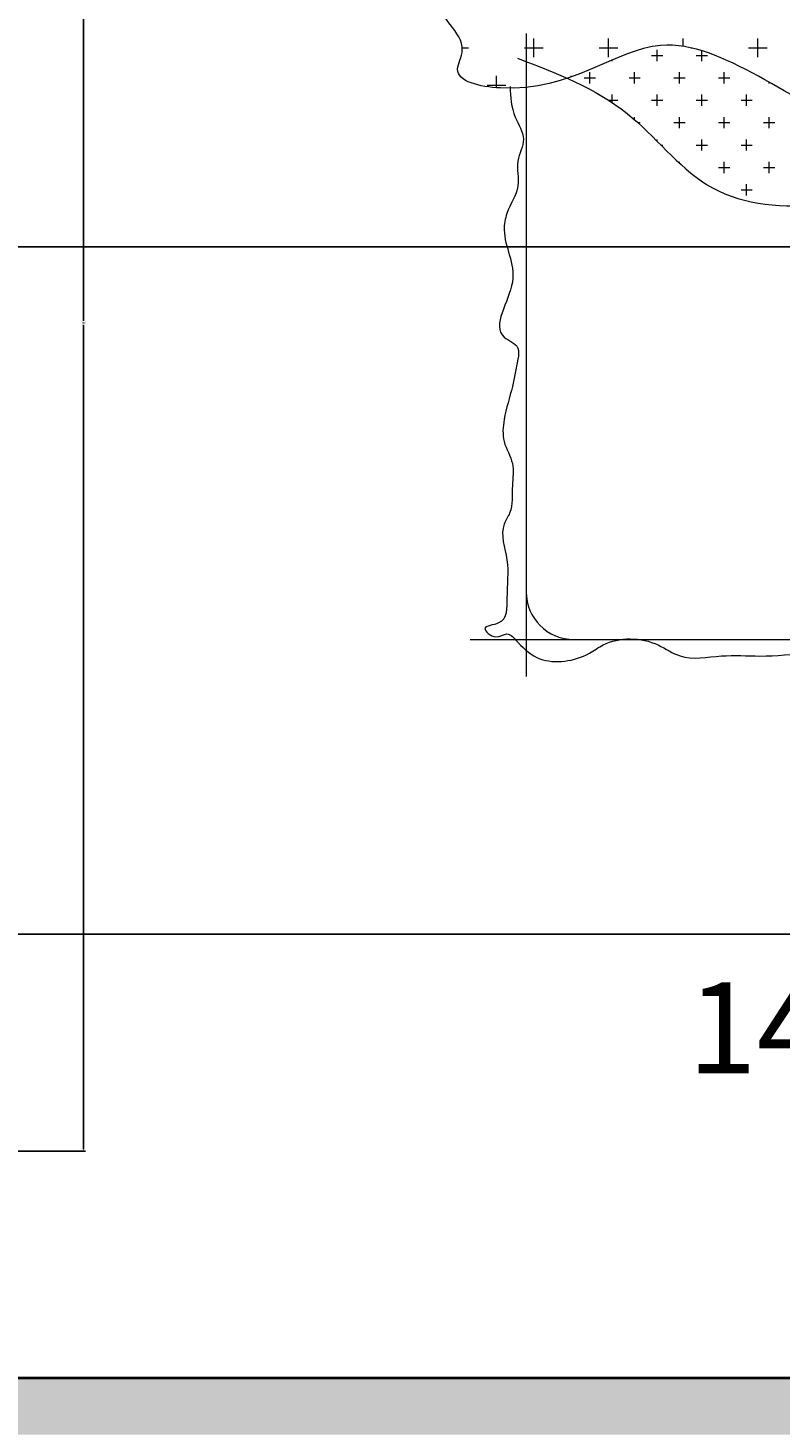
# Model space of a CAD drawing. Units: inches. Extents: x 2330 to 3943, y 1763 to 3461.
# Tile 31 of 40: x 3281 to 3347, y 2975 to 3098. Entities that reach past the tile are written whole.
import ezdxf

# ---------------------------------------------------------------- set-up
doc = ezdxf.new("R2010")
doc.units = ezdxf.units.IN
for name, color, linetype, lineweight in [('A-ANNO-DIMS', 2, 'Continuous', 18), ('A-AREA-IDEN', 7, 'Continuous', 18), ('A-FURN', 8, 'Continuous', 13), ('A-WALL', 7, 'Continuous', 40), ('A-WALL-PATT', 252, 'Continuous', 13)]:
    doc.layers.add(name, color=color, linetype=linetype, lineweight=lineweight)
doc.styles.get("Standard").update_dxf_attribs({"font": 'arial.ttf'})
doc.dimstyles.get("Standard").update_dxf_attribs({"dimtxt": 0.18, "dimasz": 0.18, "dimexe": 0.18, "dimexo": 0.0625, "dimgap": 0.09, "dimtad": 0, "dimtih": 1, "dimtoh": 1, "dimdec": 4, "dimzin": 0, "dimdsep": 46, "dimtxsty": 'Standard', "dimcen": 0.09, "dimadec": 0, "dimazin": 0, "dimtfac": 1, "dimtdec": 4, "dimtofl": 0, "dimtmove": 0, "dimatfit": 3, "dimfxl": 1, "dimtolj": 1, "dimtzin": 0, "dimarcsym": 0})

# ---------------------------------------------------------------- blocks, each defined once
blk = doc.blocks.new('A$C200C7901')
for p, q in [((0.5, 1.3845), (0.5, 0.3086)), ((0.3931, 1.3602), (0.4035, 1.3602)), ((0.3931, 1.3602), (0.4035, 1.3602)), ((0.4972, 1.3602), (0.5285, 1.3602)), ((0.4972, 1.3602), (0.5285, 1.3602)), ((0.4504, 1.2936), (0.4504, 1.3133)), ((0.4504, 1.2936), (0.4504, 1.3133)), ((0.4347, 1.2977), (0.466, 1.2977)), ((0.4347, 1.2977), (0.466, 1.2977)), ((0.4061, 0.3703), (2.0386, 0.3703))]:
    blk.add_line(p, q)
at = {"linetype": 'ByBlock'}
for p, q in [((0.5129, 1.3445), (0.5129, 1.3758)), ((0.5129, 1.3445), (0.5129, 1.3758)), ((0.6222, 1.3602), (0.6535, 1.3602)), ((0.6222, 1.3602), (0.6535, 1.3602)), ((0.6379, 1.3445), (0.6379, 1.3758)), ((0.6379, 1.3445), (0.6379, 1.3758)), ((0.7629, 1.3627), (0.7629, 1.3758)), ((0.7629, 1.3627), (0.7629, 1.3758)), ((0.7762, 1.3602), (0.7785, 1.3602)), ((0.7762, 1.3602), (0.7785, 1.3602)), ((0.8722, 1.3602), (0.9035, 1.3602)), ((0.8722, 1.3602), (0.9035, 1.3602)), ((0.8879, 1.3445), (0.8879, 1.3758)), ((0.8879, 1.3445), (0.8879, 1.3758)), ((0.6441, 1.3383), (0.6441, 1.3399)), ((0.6441, 1.3383), (0.6441, 1.3399)), ((0.7097, 1.3477), (0.7285, 1.3477)), ((0.7097, 1.3477), (0.7285, 1.3477)), ((0.7191, 1.3383), (0.7191, 1.357)), ((0.7191, 1.3383), (0.7191, 1.357)), ((0.7847, 1.3477), (0.8035, 1.3477)), ((0.7847, 1.3477), (0.8035, 1.3477)), ((0.7941, 1.3383), (0.7941, 1.3554)), ((0.7941, 1.3383), (0.7941, 1.3554)), ((0.5754, 1.3115), (0.5754, 1.3133)), ((0.5754, 1.3115), (0.5754, 1.3133)), ((0.6066, 1.3008), (0.6066, 1.3195)), ((0.6066, 1.3008), (0.6066, 1.3195)), ((0.6816, 1.3008), (0.6816, 1.3195)), ((0.6816, 1.3008), (0.6816, 1.3195)), ((0.7566, 1.3008), (0.7566, 1.3195)), ((0.7566, 1.3008), (0.7566, 1.3195)), ((0.8316, 1.3008), (0.8316, 1.3195)), ((0.8316, 1.3008), (0.8316, 1.3195)), ((0.5972, 1.3102), (0.616, 1.3102)), ((0.5972, 1.3102), (0.616, 1.3102)), ((0.6722, 1.3102), (0.691, 1.3102)), ((0.6722, 1.3102), (0.691, 1.3102)), ((0.7472, 1.3102), (0.766, 1.3102)), ((0.7472, 1.3102), (0.766, 1.3102)), ((0.8222, 1.3102), (0.841, 1.3102)), ((0.8222, 1.3102), (0.841, 1.3102)), ((0.9066, 1.3008), (0.9066, 1.3028)), ((0.9066, 1.3008), (0.9066, 1.3028)), ((0.6379, 1.2727), (0.6535, 1.2727)), ((0.6379, 1.2727), (0.6535, 1.2727)), ((0.6441, 1.2686), (0.6441, 1.282)), ((0.6441, 1.2686), (0.6441, 1.282)), ((0.7097, 1.2727), (0.7285, 1.2727)), ((0.7097, 1.2727), (0.7285, 1.2727)), ((0.7191, 1.2633), (0.7191, 1.282)), ((0.7191, 1.2633), (0.7191, 1.282)), ((0.7847, 1.2727), (0.8035, 1.2727)), ((0.7847, 1.2727), (0.8035, 1.2727)), ((0.7941, 1.2633), (0.7941, 1.282)), ((0.7941, 1.2633), (0.7941, 1.282)), ((0.8597, 1.2727), (0.8785, 1.2727)), ((0.8597, 1.2727), (0.8785, 1.2727)), ((0.8691, 1.2633), (0.8691, 1.282)), ((0.8691, 1.2633), (0.8691, 1.282)), ((0.6816, 1.2398), (0.6816, 1.2445)), ((0.6816, 1.2398), (0.6816, 1.2445)), ((0.7566, 1.2258), (0.7566, 1.2445)), ((0.7566, 1.2258), (0.7566, 1.2445)), ((0.8316, 1.2258), (0.8316, 1.2445)), ((0.8316, 1.2258), (0.8316, 1.2445)), ((0.9066, 1.2258), (0.9066, 1.2445)), ((0.9066, 1.2258), (0.9066, 1.2445)), ((0.6868, 1.2352), (0.691, 1.2352)), ((0.6868, 1.2352), (0.691, 1.2352)), ((0.7472, 1.2352), (0.766, 1.2352)), ((0.7472, 1.2352), (0.766, 1.2352)), ((0.8222, 1.2352), (0.841, 1.2352)), ((0.8222, 1.2352), (0.841, 1.2352)), ((0.8972, 1.2352), (0.916, 1.2352)), ((0.8972, 1.2352), (0.916, 1.2352)), ((0.7191, 1.2041), (0.7191, 1.207)), ((0.7191, 1.2041), (0.7191, 1.207)), ((0.7255, 1.1977), (0.7285, 1.1977)), ((0.7255, 1.1977), (0.7285, 1.1977)), ((0.7847, 1.1977), (0.8035, 1.1977)), ((0.7847, 1.1977), (0.8035, 1.1977)), ((0.7941, 1.1883), (0.7941, 1.207)), ((0.7941, 1.1883), (0.7941, 1.207)), ((0.8597, 1.1977), (0.8785, 1.1977)), ((0.8597, 1.1977), (0.8785, 1.1977)), ((0.8691, 1.1883), (0.8691, 1.207)), ((0.8691, 1.1883), (0.8691, 1.207)), ((0.7566, 1.1674), (0.7566, 1.1695)), ((0.7566, 1.1674), (0.7566, 1.1695)), ((0.7646, 1.1602), (0.766, 1.1602)), ((0.7646, 1.1602), (0.766, 1.1602)), ((0.8222, 1.1602), (0.841, 1.1602)), ((0.8222, 1.1602), (0.841, 1.1602)), ((0.8316, 1.1508), (0.8316, 1.1695)), ((0.8316, 1.1508), (0.8316, 1.1695)), ((0.8972, 1.1602), (0.916, 1.1602)), ((0.8972, 1.1602), (0.916, 1.1602)), ((0.9066, 1.1508), (0.9066, 1.1695)), ((0.9066, 1.1508), (0.9066, 1.1695)), ((0.8691, 1.1133), (0.8691, 1.132)), ((0.8691, 1.1133), (0.8691, 1.132)), ((0.8597, 1.1227), (0.8785, 1.1227)), ((0.8597, 1.1227), (0.8785, 1.1227))]:
    blk.add_line(p, q, dxfattribs=at)
blk.add_arc((0.58, 0.4503), 0.08, 180, 270)
for points, knots in [([(0.4485, 1.7835), (0.4321, 1.7496), (0.4062, 1.6964), (0.49, 1.6713), (0.4719, 1.5969), (0.4123, 1.592), (0.4233, 1.5337), (0.4954, 1.5086), (0.4012, 1.4738), (0.3253, 1.4306), (0.4113, 1.3764), (0.3688, 1.3065), (0.5579, 1.2663), (0.741, 1.4533), (1.1127, 1.1109), (1.4811, 1.2478), (1.7885, 1.3492), (2.0357, 1.1637), (2.0748, 1.2974), (2.0876, 1.349), (2.0192, 1.3805), (2.0564, 1.4298), (2.0588, 1.4846), (1.9759, 1.5349), (2.1004, 1.5845), (2.0397, 1.6519), (1.971, 1.7053), (2.1104, 1.8981), (1.5946, 1.7967), (1.2448, 1.7472), (0.8129, 1.7935), (0.4953, 1.8548), (0.4582, 1.7983), (0.4485, 1.7835)], [0, 0, 0, 0, 88.420092, 139.08588, 204.302936, 239.695496, 287.801042, 327.365471, 412.960499, 463.626286, 552.059846, 584.668336, 662.614915, 940.993281, 1309.926334, 1844.022653, 1996.276242, 2316.43048, 2341.441004, 2404.707416, 2449.463774, 2514.680778, 2538.40571, 2613.031547, 2697.13096, 2760.903931, 2822.692699, 2945.47, 3215.060018, 3725.584917, 4361.974444, 4504.671998, 4555.32777, 4555.32777, 4555.32777, 4555.32777]), ([(0.4856, 1.3429), (0.5504, 1.3182), (0.6715, 1.2721), (0.8374, 1.0498), (1.1164, 1.1183), (1.3878, 1.1816), (1.5888, 1.1102), (1.8403, 1.1127), (1.9415, 1.2178), (2.0032, 1.2819)], [0, 0, 0, 0, 205.411753, 383.654933, 772.067458, 921.644661, 1226.793228, 1388.983508, 1642.292305, 1642.292305, 1642.292305, 1642.292305])]:
    blk.add_open_spline(points, degree=3, knots=knots)
blk.add_open_spline([(0.473, 1.2954), (0.4739, 1.2781), (0.4755, 1.2477), (0.5032, 1.2084), (0.4801, 1.1701), (0.4928, 1.1255), (0.4674, 1.0912), (0.4579, 1.0351), (0.501, 0.9724), (0.4311, 0.8832), (0.4902, 0.8637), (0.4843, 0.8288), (0.4774, 0.7906), (0.4625, 0.7457), (0.459, 0.6999), (0.4816, 0.6664), (0.4748, 0.625), (0.4791, 0.5889), (0.4533, 0.5528), (0.4738, 0.5004), (0.4658, 0.4502), (0.4696, 0.3946), (0.4189, 0.3935), (0.4493, 0.3684), (0.4694, 0.3857), (0.4922, 0.3576), (0.5297, 0.3262), (0.5917, 0.3353), (0.6454, 0.3754), (0.7083, 0.3741), (0.7643, 0.3328), (0.826, 0.346), (0.925, 0.3388), (1.0353, 0.3593), (1.1561, 0.3744), (1.2477, 0.3154), (1.3302, 0.3474), (1.4086, 0.3512), (1.5217, 0.3878), (1.6362, 0.3176), (1.7682, 0.3285), (1.8402, 0.3019), (1.9071, 0.3529), (1.9647, 0.3412), (2.0795, 0.2948), (2.0472, 0.3498), (2.0343, 0.3772), (2.0435, 0.43), (2.0109, 0.5782), (2.0746, 0.4643), (2.0805, 0.584), (2.0084, 0.5979), (2.0343, 0.6846), (2.0344, 0.746), (2.0293, 0.8096), (2.0489, 0.8545), (2.0652, 0.9218), (1.9842, 0.9297), (2.0007, 1.0162), (2.0367, 1.0585), (2.0367, 1.1102), (2.0457, 1.1647), (2.0226, 1.2084), (2.0234, 1.2306), (2.0236, 1.2352)], degree=3, knots=[0, 0, 0, 0, 51.660678, 90.967412, 128.902454, 170.303599, 219.852997, 247.834962, 336.321557, 429.35469, 458.821847, 477.222321, 524.135809, 581.038434, 617.839381, 657.146115, 693.947125, 740.178081, 760.753248, 820.731705, 885.133458, 928.777044, 953.563729, 976.574207, 995.553042, 1018.563482, 1064.584401, 1147.951297, 1174.787598, 1266.851571, 1308.018447, 1377.066427, 1441.511314, 1608.245014, 1714.11869, 1792.771707, 1913.247991, 1954.931389, 2029.864445, 2259.189419, 2305.221512, 2429.507982, 2456.344283, 2543.92595, 2627.925037, 2662.96218, 2687.736879, 2719.937755, 2839.540991, 2875.47895, 2953.681041, 2993.270313, 3066.872333, 3154.395764, 3200.397042, 3248.426375, 3312.828127, 3347.881398, 3444.484026, 3481.577522, 3518.665244, 3592.267265, 3644.719162, 3658.519501, 3658.519501, 3658.519501, 3658.519501], dxfattribs=at)
blk = doc.blocks.new('*D48')
at = {"layer": 'A-ANNO-DIMS', "color": 0, "lineweight": -2, "transparency": 16777216}
for p, q in [((3262.1, 3145.15), (3286.25, 3145.15)), ((3286.07, 3144.97), (3286.07, 3072.54)), ((3286.07, 2999.75), (3286.07, 3072.18)), ((3262.1, 2999.57), (3286.25, 2999.57))]:
    blk.add_line(p, q, dxfattribs=at)
at = {"layer": 'A-ANNO-DIMS', "color": 0, "transparency": 16777216}
for points in [[(3286.04, 3144.97), (3286.1, 3144.97), (3286.07, 3145.15)], [(3286.04, 2999.75), (3286.1, 2999.75), (3286.07, 2999.57)]]:
    blk.add_solid(points, dxfattribs=at)
at = {"layer": 'Defpoints', "color": 0, "transparency": 16777216}
for p in [(3262.04, 3145.15), (3286.07, 3145.15), (3262.04, 2999.57)]:
    blk.add_point(p, dxfattribs=at)
at = {"layer": 'A-ANNO-DIMS', "color": 0, "transparency": 16777216, "insert": (3286.07, 3072.36), "char_height": 0.18, "attachment_point": 5}
blk.add_mtext('\\A1;146', dxfattribs=at)
blk = doc.blocks.new('*D86')
at = {"layer": 'A-ANNO-DIMS', "color": 0, "lineweight": -2, "transparency": 16777216}
for p, q in [((2979.18, 3100.04), (3942.54, 3100.04)), ((3942.36, 3099.86), (3942.36, 3089.72)), ((3942.36, 3079.22), (3942.36, 3089.36)), ((2979.18, 3079.04), (3942.54, 3079.04))]:
    blk.add_line(p, q, dxfattribs=at)
at = {"layer": 'A-ANNO-DIMS', "color": 0, "transparency": 16777216}
for points in [[(3942.33, 3099.86), (3942.39, 3099.86), (3942.36, 3100.04)], [(3942.33, 3079.22), (3942.39, 3079.22), (3942.36, 3079.04)]]:
    blk.add_solid(points, dxfattribs=at)
at = {"layer": 'Defpoints', "color": 0, "transparency": 16777216}
for p in [(2979.12, 3100.04), (2979.12, 3079.04), (3942.36, 3079.04)]:
    blk.add_point(p, dxfattribs=at)
at = {"layer": 'A-ANNO-DIMS', "color": 0, "transparency": 16777216, "insert": (3942.36, 3089.54), "char_height": 0.18, "attachment_point": 5}
blk.add_mtext('\\A1;21', dxfattribs=at)
blk = doc.blocks.new('*D93')
at = {"layer": 'A-ANNO-DIMS', "color": 0, "lineweight": -2, "transparency": 16777216}
for p, q in [((3446.6, 3018.65), (2330.5, 3018.65)), ((2330.68, 3018.47), (2330.68, 2999.33)), ((2330.68, 2979.83), (2330.68, 2998.97)), ((3446.6, 2979.65), (2330.5, 2979.65))]:
    blk.add_line(p, q, dxfattribs=at)
at = {"layer": 'A-ANNO-DIMS', "color": 0, "transparency": 16777216}
for points in [[(2330.65, 3018.47), (2330.71, 3018.47), (2330.68, 3018.65)], [(2330.65, 2979.83), (2330.71, 2979.83), (2330.68, 2979.65)]]:
    blk.add_solid(points, dxfattribs=at)
at = {"layer": 'Defpoints', "color": 0, "transparency": 16777216}
for p in [(2330.68, 3018.65), (3446.66, 3018.65), (3446.66, 2979.65)]:
    blk.add_point(p, dxfattribs=at)
at = {"layer": 'A-ANNO-DIMS', "color": 0, "transparency": 16777216, "insert": (2330.68, 2999.15), "char_height": 0.18, "attachment_point": 5}
blk.add_mtext('\\A1;39', dxfattribs=at)

msp = doc.modelspace()

# ---------------------------------------------------------------- hatches: boundary and pattern name
at = {"layer": 'A-WALL-PATT'}
h = msp.add_hatch(color=256, dxfattribs=at)
h.dxf.hatch_style = 1
h.paths.add_polyline_path([(3241.6605, 2974.6524), (3376.7746, 2974.6524, -0.16828569), (3398.3014, 2935.4254), (3407.174, 2936.9344, 0.12044914), (3392.5913, 2970.6524), (3455.6605, 2970.6524), (3455.6605, 3018.6524), (3446.6605, 3018.6524), (3446.6605, 2979.6524), (3275.6605, 2979.6524), (3275.6605, 3018.6524), (3270.6605, 3018.6524), (3270.6605, 2979.6524), (3154.6605, 2979.6524), (3154.6605, 2918.1524), (3150.6605, 2918.1524), (3150.6605, 2913.1524), (3154.6605, 2913.1524), (3154.6605, 2863.6524), (3159.6605, 2863.6524), (3159.6605, 2867.6524), (3196.6605, 2867.6524), (3196.6605, 2872.6524), (3159.6605, 2872.6524), (3159.6605, 2974.6524), (3236.6605, 2974.6524), (3236.6605, 2906.6524), (3241.6605, 2906.6524)])

# ---------------------------------------------------------------- linework, layer by layer
at = {"layer": 'A-WALL'}
msp.add_line((3275.6605, 2979.6524), (3446.6605, 2979.6524), dxfattribs=at)

# ---------------------------------------------------------------- block references
at = {"layer": 'A-FURN', "xscale": 52.5181391560459, "yscale": 52.5181391560459, "zscale": 52.5181391560459}
msp.add_blockref('A$C200C7901', (3298.7219, 3025.0763), dxfattribs=at)

# ---------------------------------------------------------------- texts
at = {"layer": 'A-AREA-IDEN', "insert": (3339.1901, 3014.4043), "char_height": 8, "attachment_point": 1}
msp.add_mtext_dynamic_manual_height_columns('14\'-3"X14\'-6"', width=95.491359, gutter_width=12.5, heights=[0], dxfattribs=at)

# ---------------------------------------------------------------- dimensions: what is measured, and where the dimension line sits
at = {"layer": 'A-ANNO-DIMS'}
for base, p1, p2, picture, middle in [((3286.0727, 3145.1485), (3262.0412, 2999.5664), (3262.0412, 3145.1485), '*D48', (3286.0727, 3072.3575)), ((3942.361, 3079.0386), (2979.1218, 3100.0386), (2979.1218, 3079.0386), '*D86', (3942.361, 3089.5386)), ((2330.6824, 3018.6524), (3446.6605, 2979.6524), (3446.6605, 3018.6524), '*D93', (2330.6824, 2999.1524))]:
    dim = msp.add_linear_dim(base=base, p1=p1, p2=p2, angle=90, dimstyle='Standard', override={"dimdec": 0, "dimlfac": 1, "dimrnd": 0, "dimzin": 0, "dimdsep": 46, "dimlunit": 2}, dxfattribs=at)
    dim.commit()
    dim.dimension.update_dxf_attribs({"geometry": picture, "text_midpoint": middle})

doc.saveas('drawing.dxf')
